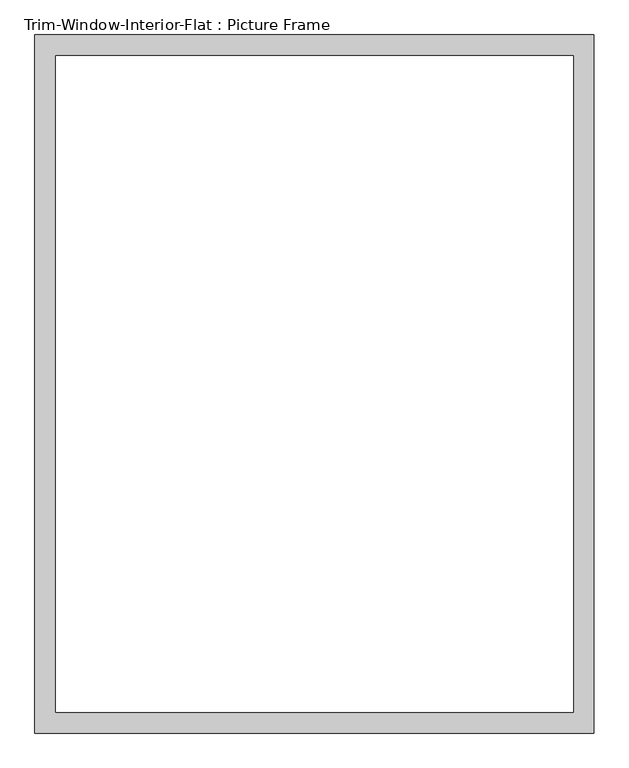
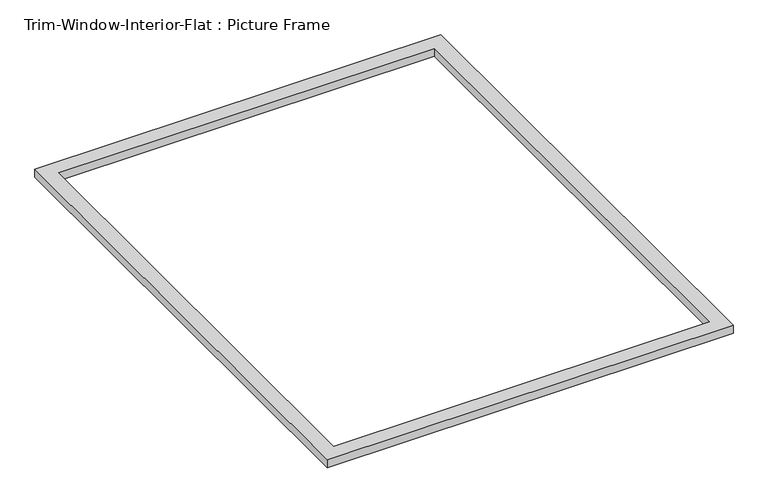
"""IFC4 building model written with IfcOpenShell, lengths in millimetres: proxy geometry, Trim-Window-Interior-Flat : Picture Frame."""

from ifc_helpers import new_model, si_unit, origin, origin_with_axes, place, context, project, spatial, polyline, outline, extrude, source, transform, mapped, element, save


def trim_window_interior_flat_picture_frame_2a7685fe(model_context):
    return source(origin(), model_context, "Body", "SweptSolid", [
        extrude(outline(polyline([(768.35, 44.45), (768.35, -1873.25), (-768.35, -1873.25), (-768.35, 44.45), (768.35, 44.45)]), holes=[polyline([(711.2, -12.7), (-711.2, -12.7), (-711.2, -1816.1), (711.2, -1816.1), (711.2, -12.7)])]), origin_with_axes(), (0.0, 0.0, 1.0), 31.75),
    ])


if __name__ == "__main__":
    model = new_model("IFC4")
    model_context = context("Model", 3, world=origin())
    ifc_project = project(units=[si_unit("LENGTHUNIT", "METRE", prefix="MILLI")], contexts=[model_context])
    site = spatial("IfcSite", under=ifc_project)
    building = spatial("IfcBuilding", under=site)
    placement = place(None, origin())
    trim_window_interior_flat_picture_frame_shape = trim_window_interior_flat_picture_frame_2a7685fe(model_context)
    element("IfcBuildingElementProxy", 1, Name="Trim-Window-Interior-Flat : Picture Frame", ObjectType="Trim-Window-Interior-Flat : Picture Frame", at=placement, inside=building, context=model_context, shape_type="MappedRepresentation", body=[
        mapped(trim_window_interior_flat_picture_frame_shape, transform((0.0, 0.0, 0.0), x_axis=(1.0, 0.0, 0.0), y_axis=(0.0, 1.0, 0.0), z_axis=(0.0, 0.0, 1.0))),
    ])
    save(model, "model.ifc")

# Revit data of these elements
# Type "Trim-Window-Interior-Flat : Picture Frame"
#   Trim Thickness_Picture Frame = 0' - 1 1/4"
#   Trim Width = 0' - 2 1/4"
#   Trim Thickness_with Sill = 0' - 0 3/4"
#   Sill Thickness = 0' - 1 1/4"
#   Opening Width [instance default] = 2' - 0"
#   Opening Height [instance default] = 3' - 0"
#   Default Elevation = 4' - 0"
#   Sill = no
#   Picture Frame = yes
#   Trim Material [instance default] = none
# Element 1 (IfcBuildingElementProxy, "Trim-Window-Interior-Flat : Picture Frame")
#   Opening Width = 4' - 9"
#   Opening Height = 6' - 0"
#   Trim Material = Wood - Stained
#   Materials on its faces: "Wood - Stained"
# Materials
#   "Wood - Stained": class "Wood", colour RGB 224 178 126, transparency 0, Cost = 0
